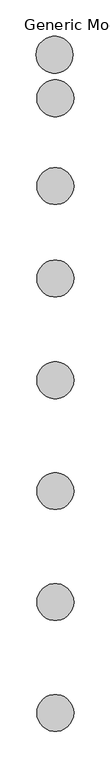
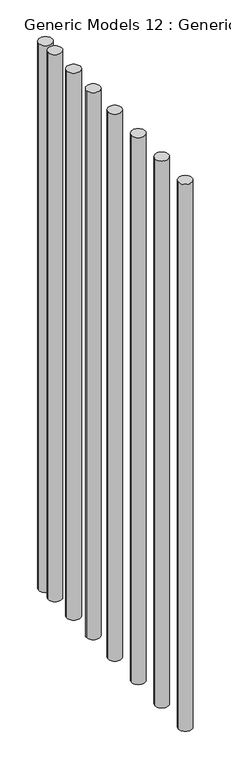
"""IFC4 building model written with IfcOpenShell, lengths in millimetres: proxy geometry, Generic Models 12 : Generic Models 12."""

from ifc_helpers import new_model, si_unit, point, frame, frame_2d, origin, place, context, project, spatial, circle_curve, trimmed, segment, composite_curve, outline, extrude, source, transform, mapped, element, save


def generic_models_12_generic_models_12_e0019dea(model_context):
    return source(origin(), model_context, "Body", "SweptSolid", [
        extrude(outline(composite_curve([segment(trimmed(circle_curve(frame_2d((-4880.4966301, -2495.9430806)), 25.4), [point((-4905.8966301, -2495.9430806))], [point((-4855.0966301, -2495.9430806))], False, "CARTESIAN"), True, "CONTINUOUS"), segment(trimmed(circle_curve(frame_2d((-4880.4966301, -2495.9430806)), 25.4), [point((-4855.0966301, -2495.9430806))], [point((-4905.8966301, -2495.9430806))], False, "CARTESIAN"), True, "CONTINUOUS")], self_intersect=False)), frame((0.0, 0.0, 7924.8), z_axis=(0.0, 0.0, 1.0), x_axis=(1.0, 0.0, 0.0)), (0.0, 0.0, 1.0), 2159.2865995),
        extrude(outline(composite_curve([segment(trimmed(circle_curve(frame_2d((-4880.4966301, -2343.5430806)), 25.4), [point((-4905.8966301, -2343.5430806))], [point((-4855.0966301, -2343.5430806))], False, "CARTESIAN"), True, "CONTINUOUS"), segment(trimmed(circle_curve(frame_2d((-4880.4966301, -2343.5430806)), 25.4), [point((-4855.0966301, -2343.5430806))], [point((-4905.8966301, -2343.5430806))], False, "CARTESIAN"), True, "CONTINUOUS")], self_intersect=False)), frame((0.0, 0.0, 7924.8), z_axis=(0.0, 0.0, 1.0), x_axis=(1.0, 0.0, 0.0)), (0.0, 0.0, 1.0), 2159.2865995),
        extrude(outline(composite_curve([segment(trimmed(circle_curve(frame_2d((-4880.4966301, -2191.1430806)), 25.4), [point((-4905.8966301, -2191.1430806))], [point((-4855.0966301, -2191.1430806))], False, "CARTESIAN"), True, "CONTINUOUS"), segment(trimmed(circle_curve(frame_2d((-4880.4966301, -2191.1430806)), 25.4), [point((-4855.0966301, -2191.1430806))], [point((-4905.8966301, -2191.1430806))], False, "CARTESIAN"), True, "CONTINUOUS")], self_intersect=False)), frame((0.0, 0.0, 7924.8), z_axis=(0.0, 0.0, 1.0), x_axis=(1.0, 0.0, 0.0)), (0.0, 0.0, 1.0), 2159.2865995),
        extrude(outline(composite_curve([segment(trimmed(circle_curve(frame_2d((-4880.4966301, -2038.7430806)), 25.4), [point((-4905.8966301, -2038.7430806))], [point((-4855.0966301, -2038.7430806))], False, "CARTESIAN"), True, "CONTINUOUS"), segment(trimmed(circle_curve(frame_2d((-4880.4966301, -2038.7430806)), 25.4), [point((-4855.0966301, -2038.7430806))], [point((-4905.8966301, -2038.7430806))], False, "CARTESIAN"), True, "CONTINUOUS")], self_intersect=False)), frame((0.0, 0.0, 7924.8), z_axis=(0.0, 0.0, 1.0), x_axis=(1.0, 0.0, 0.0)), (0.0, 0.0, 1.0), 2159.2865995),
        extrude(outline(composite_curve([segment(trimmed(circle_curve(frame_2d((-4880.4966301, -1899.0430806)), 25.4), [point((-4905.8966301, -1899.0430806))], [point((-4855.0966301, -1899.0430806))], False, "CARTESIAN"), True, "CONTINUOUS"), segment(trimmed(circle_curve(frame_2d((-4880.4966301, -1899.0430806)), 25.4), [point((-4855.0966301, -1899.0430806))], [point((-4905.8966301, -1899.0430806))], False, "CARTESIAN"), True, "CONTINUOUS")], self_intersect=False)), frame((0.0, 0.0, 7924.8), z_axis=(0.0, 0.0, 1.0), x_axis=(1.0, 0.0, 0.0)), (0.0, 0.0, 1.0), 2159.2865995),
        extrude(outline(composite_curve([segment(trimmed(circle_curve(frame_2d((-4880.4966301, -1772.0430806)), 25.4), [point((-4905.8966301, -1772.0430806))], [point((-4855.0966301, -1772.0430806))], False, "CARTESIAN"), True, "CONTINUOUS"), segment(trimmed(circle_curve(frame_2d((-4880.4966301, -1772.0430806)), 25.4), [point((-4855.0966301, -1772.0430806))], [point((-4905.8966301, -1772.0430806))], False, "CARTESIAN"), True, "CONTINUOUS")], self_intersect=False)), frame((0.0, 0.0, 7924.8), z_axis=(0.0, 0.0, 1.0), x_axis=(1.0, 0.0, 0.0)), (0.0, 0.0, 1.0), 2159.2865995),
        extrude(outline(composite_curve([segment(trimmed(circle_curve(frame_2d((-4880.4966301, -1651.3930806)), 25.4), [point((-4905.8966301, -1651.3930806))], [point((-4855.0966301, -1651.3930806))], False, "CARTESIAN"), True, "CONTINUOUS"), segment(trimmed(circle_curve(frame_2d((-4880.4966301, -1651.3930806)), 25.4), [point((-4855.0966301, -1651.3930806))], [point((-4905.8966301, -1651.3930806))], False, "CARTESIAN"), True, "CONTINUOUS")], self_intersect=False)), frame((0.0, 0.0, 7924.8), z_axis=(0.0, 0.0, 1.0), x_axis=(1.0, 0.0, 0.0)), (0.0, 0.0, 1.0), 2159.2865995),
        extrude(outline(composite_curve([segment(trimmed(circle_curve(frame_2d((-4881.3729153, -1591.6776324)), 25.4), [point((-4906.7729153, -1591.6776324))], [point((-4855.9729153, -1591.6776324))], False, "CARTESIAN"), True, "CONTINUOUS"), segment(trimmed(circle_curve(frame_2d((-4881.3729153, -1591.6776324)), 25.4), [point((-4855.9729153, -1591.6776324))], [point((-4906.7729153, -1591.6776324))], False, "CARTESIAN"), True, "CONTINUOUS")], self_intersect=False)), frame((0.0, 0.0, 7924.8), z_axis=(0.0, 0.0, 1.0), x_axis=(1.0, 0.0, 0.0)), (0.0, 0.0, 1.0), 2159.2865995),
    ])


if __name__ == "__main__":
    model = new_model("IFC4")
    model_context = context("Model", 3, world=origin())
    ifc_project = project(units=[si_unit("LENGTHUNIT", "METRE", prefix="MILLI")], contexts=[model_context])
    site = spatial("IfcSite", under=ifc_project)
    building = spatial("IfcBuilding", under=site)
    placement = place(None, origin())
    generic_models_12_generic_models_12_shape = generic_models_12_generic_models_12_e0019dea(model_context)
    element("IfcBuildingElementProxy", 1, Name="Generic Models 12 : Generic Models 12", ObjectType="Generic Models 12 : Generic Models 12", at=placement, inside=building, context=model_context, shape_type="MappedRepresentation", body=[
        mapped(generic_models_12_generic_models_12_shape, transform((0.0, 0.0, 0.0), x_axis=(1.0, 0.0, 0.0), y_axis=(0.0, 1.0, 0.0), z_axis=(0.0, 0.0, 1.0))),
    ])
    save(model, "model.ifc")
